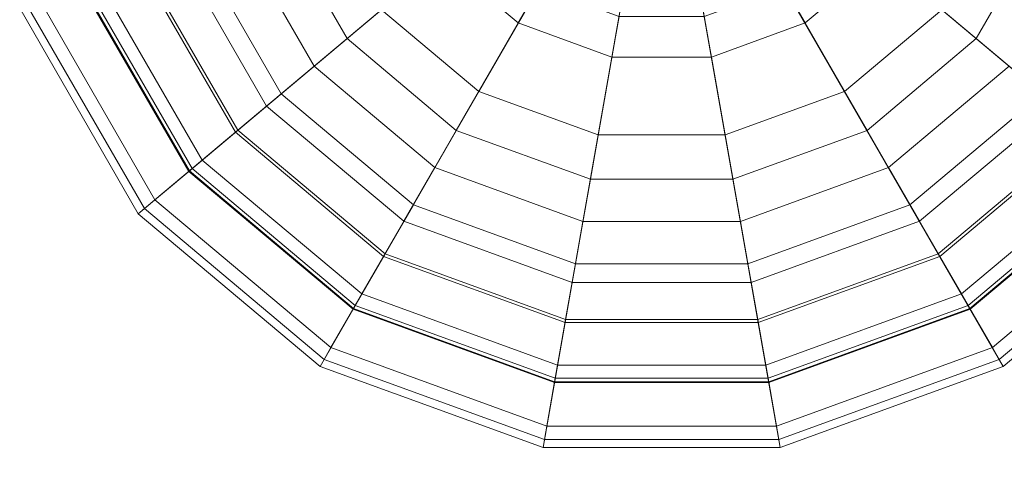
# Model space of a CAD drawing. Units: inches. Extents: x 375 to 1122, y 27 to 1069.
# Tile 30 of 155: x 731.789 to 733.741, y 279.842 to 280.756. Entities that reach past the tile are written whole.
import ezdxf

# ---------------------------------------------------------------- set-up
doc = ezdxf.new("R2010")
doc.units = ezdxf.units.IN
doc.layers.add('A-ANNO-DIMS', color=2, linetype='Continuous', lineweight=18)
doc.layers.add('Furniture', color=30, linetype='Continuous', lineweight=18)
doc.styles.get("Standard").update_dxf_attribs({"font": 'arial.ttf'})
doc.dimstyles.new('ISO-25', dxfattribs={"dimtxt": 12, "dimasz": 2.5, "dimexe": 1.5, "dimexo": 1.5, "dimtad": 1, "dimdec": 1, "dimlunit": 3, "dimtxsty": 'Standard', "dimblk": 'ARCHTICK', "dimcen": 2.5, "dimadec": 0, "dimazin": 0, "dimtfac": 1, "dimtdec": 1, "dimtmove": 0, "dimatfit": 3, "dimfxl": 1.5, "dimfxlon": 1, "dimarcsym": 0})

# ---------------------------------------------------------------- blocks, each defined once
blk = doc.blocks.new('A$C403C54AD')
for points in [[(1.64823, 1.228857, -0.04658), (1.626464, 1.202917, -0.043501), (1.626464, 1.202917, -0.043501), (1.638046, 1.234737, -0.04658)], [(1.635601, 1.213806, -0.040074), (1.646131, 1.226356, -0.043349), (1.636929, 1.231669, -0.043349), (1.631326, 1.216274, -0.040074)], [(1.65579, 1.219849, -0.04658), (1.626464, 1.202917, -0.043501), (1.626464, 1.202917, -0.043501), (1.64823, 1.228857, -0.04658)], [(1.652961, 1.218216, -0.043349), (1.65579, 1.219849, -0.04658), (1.64823, 1.228857, -0.04658), (1.646131, 1.226356, -0.043349)], [(1.644092, 1.223925, 0.056929), (1.63955, 1.218512, 0.046697), (1.633427, 1.222047, 0.046697), (1.635844, 1.228687, 0.056929)], [(1.652926, 1.218195, 0.116404), (1.655444, 1.219649, 0.10318), (1.647974, 1.228552, 0.10318), (1.646105, 1.226325, 0.116404)], [(1.655444, 1.219649, 0.10318), (1.65486, 1.219312, 0.074938), (1.64754, 1.228035, 0.074938), (1.647974, 1.228552, 0.10318)], [(1.65486, 1.219312, 0.074938), (1.650214, 1.216629, 0.056929), (1.644092, 1.223925, 0.056929), (1.64754, 1.228035, 0.074938)], [(1.638116, 1.216804, 0.048884), (1.642285, 1.221772, 0.058276), (1.634882, 1.226046, 0.058276), (1.632664, 1.219951, 0.048884)], [(1.638774, 1.210025, -0.040074), (1.652961, 1.218216, -0.043349), (1.646131, 1.226356, -0.043349), (1.635601, 1.213806, -0.040074)], [(1.648599, 1.215697, 0.12581), (1.652926, 1.218195, 0.116404), (1.646105, 1.226325, 0.116404), (1.642894, 1.222497, 0.12581)], [(1.652773, 1.218107, 0.102963), (1.65034, 1.216702, 0.115599), (1.644185, 1.224037, 0.115599), (1.645991, 1.226189, 0.102963)], [(1.652203, 1.217778, 0.075423), (1.652773, 1.218107, 0.102963), (1.645991, 1.226189, 0.102963), (1.645568, 1.225685, 0.075423)], [(1.64778, 1.215224, 0.058276), (1.652203, 1.217778, 0.075423), (1.645568, 1.225685, 0.075423), (1.642285, 1.221772, 0.058276)], [(1.65034, 1.216702, 0.115599), (1.645933, 1.214158, 0.12581), (1.640915, 1.220139, 0.12581), (1.644185, 1.224037, 0.115599)], [(1.650214, 1.216629, 0.056929), (1.644094, 1.213096, 0.046697), (1.63955, 1.218512, 0.046697), (1.644092, 1.223925, 0.056929)], [(1.63955, 1.218512, 0.046697), (1.632968, 1.210669, 0.03933), (1.629925, 1.212426, 0.03933), (1.633427, 1.222047, 0.046697)], [(1.645933, 1.214158, 0.12581), (1.648599, 1.215697, 0.12581), (1.642894, 1.222497, 0.12581), (1.640915, 1.220139, 0.12581)], [(1.642163, 1.211981, 0.048884), (1.64778, 1.215224, 0.058276), (1.642285, 1.221772, 0.058276), (1.638116, 1.216804, 0.048884)], [(1.659812, 1.208798, -0.04658), (1.626464, 1.202917, -0.043501), (1.626464, 1.202917, -0.043501), (1.65579, 1.219849, -0.04658)], [(1.656556, 1.208223, 0.116404), (1.659419, 1.208728, 0.10318), (1.655444, 1.219649, 0.10318), (1.652926, 1.218195, 0.116404)], [(1.656596, 1.20823, -0.043349), (1.659812, 1.208798, -0.04658), (1.65579, 1.219849, -0.04658), (1.652961, 1.218216, -0.043349)], [(1.659419, 1.208728, 0.10318), (1.658754, 1.208611, 0.074938), (1.65486, 1.219312, 0.074938), (1.655444, 1.219649, 0.10318)], [(1.658754, 1.208611, 0.074938), (1.653471, 1.20768, 0.056929), (1.650214, 1.216629, 0.056929), (1.65486, 1.219312, 0.074938)], [(1.644094, 1.213096, 0.046697), (1.635227, 1.207977, 0.03933), (1.632968, 1.210669, 0.03933), (1.63955, 1.218512, 0.046697)], [(1.640462, 1.205386, -0.040074), (1.656596, 1.20823, -0.043349), (1.652961, 1.218216, -0.043349), (1.638774, 1.210025, -0.040074)], [(1.651635, 1.207356, 0.12581), (1.656556, 1.208223, 0.116404), (1.652926, 1.218195, 0.116404), (1.648599, 1.215697, 0.12581)], [(1.650703, 1.207191, 0.058276), (1.655733, 1.208078, 0.075423), (1.652203, 1.217778, 0.075423), (1.64778, 1.215224, 0.058276)], [(1.656381, 1.208193, 0.102963), (1.653614, 1.207705, 0.115599), (1.65034, 1.216702, 0.115599), (1.652773, 1.218107, 0.102963)], [(1.655733, 1.208078, 0.075423), (1.656381, 1.208193, 0.102963), (1.652773, 1.218107, 0.102963), (1.652203, 1.217778, 0.075423)], [(1.634175, 1.207369, 0.042248), (1.642163, 1.211981, 0.048884), (1.638116, 1.216804, 0.048884), (1.632188, 1.209738, 0.042248)], [(1.653614, 1.207705, 0.115599), (1.648604, 1.206821, 0.12581), (1.645933, 1.214158, 0.12581), (1.65034, 1.216702, 0.115599)], [(1.653471, 1.20768, 0.056929), (1.646512, 1.206452, 0.046697), (1.644094, 1.213096, 0.046697), (1.650214, 1.216629, 0.056929)], [(1.648604, 1.206821, 0.12581), (1.651635, 1.207356, 0.12581), (1.648599, 1.215697, 0.12581), (1.645933, 1.214158, 0.12581)], [(1.644316, 1.206065, 0.048884), (1.650703, 1.207191, 0.058276), (1.64778, 1.215224, 0.058276), (1.642163, 1.211981, 0.048884)], [(1.637001, 1.209001, -0.037209), (1.638774, 1.210025, -0.040074), (1.635601, 1.213806, -0.040074), (1.634285, 1.212238, -0.037209)], [(1.646512, 1.206452, 0.046697), (1.636429, 1.204675, 0.03933), (1.635227, 1.207977, 0.03933), (1.644094, 1.213096, 0.046697)], [(1.635233, 1.204464, 0.042248), (1.644316, 1.206065, 0.048884), (1.642163, 1.211981, 0.048884), (1.634175, 1.207369, 0.042248)], [(1.638446, 1.20503, -0.037209), (1.640462, 1.205386, -0.040074), (1.638774, 1.210025, -0.040074), (1.637001, 1.209001, -0.037209)], [(1.659812, 1.197037, -0.04658), (1.626464, 1.202917, -0.043501), (1.626464, 1.202917, -0.043501), (1.659812, 1.208798, -0.04658)], [(1.658754, 1.197224, 0.074938), (1.653471, 1.198155, 0.056929), (1.653471, 1.20768, 0.056929), (1.658754, 1.208611, 0.074938)], [(1.656556, 1.197611, 0.116404), (1.659419, 1.197107, 0.10318), (1.659419, 1.208728, 0.10318), (1.656556, 1.208223, 0.116404)], [(1.656596, 1.197604, -0.043349), (1.659812, 1.197037, -0.04658), (1.659812, 1.208798, -0.04658), (1.656596, 1.20823, -0.043349)], [(1.659419, 1.197107, 0.10318), (1.658754, 1.197224, 0.074938), (1.658754, 1.208611, 0.074938), (1.659419, 1.208728, 0.10318)], [(1.640462, 1.200449, -0.040074), (1.656596, 1.197604, -0.043349), (1.656596, 1.20823, -0.043349), (1.640462, 1.205386, -0.040074)], [(1.650703, 1.198643, 0.058276), (1.655733, 1.197756, 0.075423), (1.655733, 1.208078, 0.075423), (1.650703, 1.207191, 0.058276)], [(1.651635, 1.198479, 0.12581), (1.656556, 1.197611, 0.116404), (1.656556, 1.208223, 0.116404), (1.651635, 1.207356, 0.12581)], [(1.656381, 1.197642, 0.102963), (1.653614, 1.19813, 0.115599), (1.653614, 1.207705, 0.115599), (1.656381, 1.208193, 0.102963)], [(1.655733, 1.197756, 0.075423), (1.656381, 1.197642, 0.102963), (1.656381, 1.208193, 0.102963), (1.655733, 1.208078, 0.075423)], [(1.653471, 1.198155, 0.056929), (1.646512, 1.199382, 0.046697), (1.646512, 1.206452, 0.046697), (1.653471, 1.20768, 0.056929)], [(1.653614, 1.19813, 0.115599), (1.648604, 1.199014, 0.12581), (1.648604, 1.206821, 0.12581), (1.653614, 1.207705, 0.115599)], [(1.644316, 1.19977, 0.048884), (1.650703, 1.198643, 0.058276), (1.650703, 1.207191, 0.058276), (1.644316, 1.206065, 0.048884)], [(1.648604, 1.199014, 0.12581), (1.651635, 1.198479, 0.12581), (1.651635, 1.207356, 0.12581), (1.648604, 1.206821, 0.12581)], [(1.646512, 1.199382, 0.046697), (1.636429, 1.20116, 0.03933), (1.636429, 1.204675, 0.03933), (1.646512, 1.206452, 0.046697)], [(1.635233, 1.201371, 0.042248), (1.644316, 1.19977, 0.048884), (1.644316, 1.206065, 0.048884), (1.635233, 1.204464, 0.042248)], [(1.638446, 1.200805, -0.037209), (1.640462, 1.200449, -0.040074), (1.640462, 1.205386, -0.040074), (1.638446, 1.20503, -0.037209)], [(1.65579, 1.185986, -0.04658), (1.626464, 1.202917, -0.043501), (1.626464, 1.202917, -0.043501), (1.659812, 1.197037, -0.04658)], [(1.64823, 1.176977, -0.04658), (1.626464, 1.202917, -0.043501), (1.626464, 1.202917, -0.043501), (1.65579, 1.185986, -0.04658)], [(1.638046, 1.171097, -0.04658), (1.626464, 1.202917, -0.043501), (1.626464, 1.202917, -0.043501), (1.64823, 1.176977, -0.04658)], [(1.634175, 1.198465, 0.042248), (1.642163, 1.193854, 0.048884), (1.644316, 1.19977, 0.048884), (1.635233, 1.201371, 0.042248)], [(1.644094, 1.192739, 0.046697), (1.635227, 1.197858, 0.03933), (1.636429, 1.20116, 0.03933), (1.646512, 1.199382, 0.046697)], [(1.637001, 1.196834, -0.037209), (1.638774, 1.19581, -0.040074), (1.640462, 1.200449, -0.040074), (1.638446, 1.200805, -0.037209)], [(1.638774, 1.19581, -0.040074), (1.652961, 1.187619, -0.043349), (1.656596, 1.197604, -0.043349), (1.640462, 1.200449, -0.040074)], [(1.642163, 1.193854, 0.048884), (1.64778, 1.190611, 0.058276), (1.650703, 1.198643, 0.058276), (1.644316, 1.19977, 0.048884)], [(1.650214, 1.189206, 0.056929), (1.644094, 1.192739, 0.046697), (1.646512, 1.199382, 0.046697), (1.653471, 1.198155, 0.056929)], [(1.645933, 1.191677, 0.12581), (1.648599, 1.190138, 0.12581), (1.651635, 1.198479, 0.12581), (1.648604, 1.199014, 0.12581)], [(1.65034, 1.189133, 0.115599), (1.645933, 1.191677, 0.12581), (1.648604, 1.199014, 0.12581), (1.653614, 1.19813, 0.115599)], [(1.64778, 1.190611, 0.058276), (1.652203, 1.188057, 0.075423), (1.655733, 1.197756, 0.075423), (1.650703, 1.198643, 0.058276)], [(1.632188, 1.196096, 0.042248), (1.638116, 1.189031, 0.048884), (1.642163, 1.193854, 0.048884), (1.634175, 1.198465, 0.042248)], [(1.648599, 1.190138, 0.12581), (1.652926, 1.187639, 0.116404), (1.656556, 1.197611, 0.116404), (1.651635, 1.198479, 0.12581)], [(1.65486, 1.186523, 0.074938), (1.650214, 1.189206, 0.056929), (1.653471, 1.198155, 0.056929), (1.658754, 1.197224, 0.074938)], [(1.652773, 1.187728, 0.102963), (1.65034, 1.189133, 0.115599), (1.653614, 1.19813, 0.115599), (1.656381, 1.197642, 0.102963)], [(1.63955, 1.187323, 0.046697), (1.632968, 1.195166, 0.03933), (1.635227, 1.197858, 0.03933), (1.644094, 1.192739, 0.046697)], [(1.652203, 1.188057, 0.075423), (1.652773, 1.187728, 0.102963), (1.656381, 1.197642, 0.102963), (1.655733, 1.197756, 0.075423)], [(1.652926, 1.187639, 0.116404), (1.655444, 1.186186, 0.10318), (1.659419, 1.197107, 0.10318), (1.656556, 1.197611, 0.116404)], [(1.652961, 1.187619, -0.043349), (1.65579, 1.185986, -0.04658), (1.659812, 1.197037, -0.04658), (1.656596, 1.197604, -0.043349)], [(1.655444, 1.186186, 0.10318), (1.65486, 1.186523, 0.074938), (1.658754, 1.197224, 0.074938), (1.659419, 1.197107, 0.10318)], [(1.634285, 1.193597, -0.037209), (1.635601, 1.192029, -0.040074), (1.638774, 1.19581, -0.040074), (1.637001, 1.196834, -0.037209)], [(1.635601, 1.192029, -0.040074), (1.646131, 1.179479, -0.043349), (1.652961, 1.187619, -0.043349), (1.638774, 1.19581, -0.040074)], [(1.633427, 1.183788, 0.046697), (1.629925, 1.193409, 0.03933), (1.632968, 1.195166, 0.03933), (1.63955, 1.187323, 0.046697)], [(1.638116, 1.189031, 0.048884), (1.642285, 1.184063, 0.058276), (1.64778, 1.190611, 0.058276), (1.642163, 1.193854, 0.048884)], [(1.644092, 1.18191, 0.056929), (1.63955, 1.187323, 0.046697), (1.644094, 1.192739, 0.046697), (1.650214, 1.189206, 0.056929)], [(1.631326, 1.18956, -0.040074), (1.636929, 1.174166, -0.043349), (1.646131, 1.179479, -0.043349), (1.635601, 1.192029, -0.040074)], [(1.640915, 1.185696, 0.12581), (1.642894, 1.183338, 0.12581), (1.648599, 1.190138, 0.12581), (1.645933, 1.191677, 0.12581)], [(1.644185, 1.181798, 0.115599), (1.640915, 1.185696, 0.12581), (1.645933, 1.191677, 0.12581), (1.65034, 1.189133, 0.115599)], [(1.642285, 1.184063, 0.058276), (1.645568, 1.18015, 0.075423), (1.652203, 1.188057, 0.075423), (1.64778, 1.190611, 0.058276)], [(1.642894, 1.183338, 0.12581), (1.646105, 1.17951, 0.116404), (1.652926, 1.187639, 0.116404), (1.648599, 1.190138, 0.12581)], [(1.632664, 1.185883, 0.048884), (1.634882, 1.179789, 0.058276), (1.642285, 1.184063, 0.058276), (1.638116, 1.189031, 0.048884)], [(1.64754, 1.1778, 0.074938), (1.644092, 1.18191, 0.056929), (1.650214, 1.189206, 0.056929), (1.65486, 1.186523, 0.074938)], [(1.645991, 1.179646, 0.102963), (1.644185, 1.181798, 0.115599), (1.65034, 1.189133, 0.115599), (1.652773, 1.187728, 0.102963)], [(1.645568, 1.18015, 0.075423), (1.645991, 1.179646, 0.102963), (1.652773, 1.187728, 0.102963), (1.652203, 1.188057, 0.075423)], [(1.646105, 1.17951, 0.116404), (1.647974, 1.177283, 0.10318), (1.655444, 1.186186, 0.10318), (1.652926, 1.187639, 0.116404)], [(1.646131, 1.179479, -0.043349), (1.64823, 1.176977, -0.04658), (1.65579, 1.185986, -0.04658), (1.652961, 1.187619, -0.043349)], [(1.635844, 1.177147, 0.056929), (1.633427, 1.183788, 0.046697), (1.63955, 1.187323, 0.046697), (1.644092, 1.18191, 0.056929)], [(1.647974, 1.177283, 0.10318), (1.64754, 1.1778, 0.074938), (1.65486, 1.186523, 0.074938), (1.655444, 1.186186, 0.10318)], [(1.634153, 1.181792, 0.12581), (1.635206, 1.178899, 0.12581), (1.642894, 1.183338, 0.12581), (1.640915, 1.185696, 0.12581)], [(1.635893, 1.177011, 0.115599), (1.634153, 1.181792, 0.12581), (1.640915, 1.185696, 0.12581), (1.644185, 1.181798, 0.115599)], [(1.634882, 1.179789, 0.058276), (1.636629, 1.174989, 0.075423), (1.645568, 1.18015, 0.075423), (1.642285, 1.184063, 0.058276)], [(1.635206, 1.178899, 0.12581), (1.636915, 1.174204, 0.116404), (1.646105, 1.17951, 0.116404), (1.642894, 1.183338, 0.12581)], [(1.637678, 1.172106, 0.074938), (1.635844, 1.177147, 0.056929), (1.644092, 1.18191, 0.056929), (1.64754, 1.1778, 0.074938)], [(1.636854, 1.174371, 0.102963), (1.635893, 1.177011, 0.115599), (1.644185, 1.181798, 0.115599), (1.645991, 1.179646, 0.102963)], [(1.636629, 1.174989, 0.075423), (1.636854, 1.174371, 0.102963), (1.645991, 1.179646, 0.102963), (1.645568, 1.18015, 0.075423)], [(1.636915, 1.174204, 0.116404), (1.637909, 1.171472, 0.10318), (1.647974, 1.177283, 0.10318), (1.646105, 1.17951, 0.116404)], [(1.636929, 1.174166, -0.043349), (1.638046, 1.171097, -0.04658), (1.64823, 1.176977, -0.04658), (1.646131, 1.179479, -0.043349)], [(1.637909, 1.171472, 0.10318), (1.637678, 1.172106, 0.074938), (1.64754, 1.1778, 0.074938), (1.647974, 1.177283, 0.10318)]]:
    blk.add_3dface(points)
blk = doc.blocks.new('_ArchTick')
at = {"color": 0, "linetype": 'ByBlock', "const_width": 0.15}
blk.add_lwpolyline([(-0.5, -0.5), (0.5, 0.5)], dxfattribs=at)
blk = doc.blocks.new('*D94')
at = {"layer": 'A-ANNO-DIMS', "color": 0, "lineweight": -2, "transparency": 16777216}
for p, q in [((734.0073, 117.5277), (734.0073, 114.5277)), ((773.0073, 117.5277), (773.0073, 114.5277)), ((734.0073, 116.0277), (773.0073, 116.0277))]:
    blk.add_line(p, q, dxfattribs=at)
at = {"layer": 'Defpoints', "color": 0, "transparency": 16777216}
for p in [(734.0073, 667.5277), (773.0073, 667.5277), (773.0073, 116.0277)]:
    blk.add_point(p, dxfattribs=at)
at = {"layer": 'A-ANNO-DIMS', "color": 0, "lineweight": -2, "transparency": 16777216, "xscale": 2.5, "yscale": 2.5, "zscale": 2.5, "rotation": 180}
blk.add_blockref('_ArchTick', (734.0073, 116.0277), dxfattribs=at)
at = {"layer": 'A-ANNO-DIMS', "color": 0, "lineweight": -2, "transparency": 16777216, "xscale": 2.5, "yscale": 2.5, "zscale": 2.5}
blk.add_blockref('_ArchTick', (773.0073, 116.0277), dxfattribs=at)
at = {"layer": 'A-ANNO-DIMS', "color": 0, "transparency": 16777216, "insert": (753.5073, 122.7837), "char_height": 12, "attachment_point": 5}
blk.add_mtext('3\'-3"', dxfattribs=at)

msp = doc.modelspace()

# ---------------------------------------------------------------- block references
at = {"layer": 'Furniture', "xscale": 39.9918517141215, "yscale": 39.9918517141215, "zscale": 39.9918517141215, "rotation": 270}
msp.add_blockref('A$C403C54AD', (684.9549, 346.2875, 0.024), dxfattribs=at)

# ---------------------------------------------------------------- dimensions: what is measured, and where the dimension line sits
at = {"layer": 'A-ANNO-DIMS'}
dim = msp.add_linear_dim(base=(773.0073, 116.0277), p1=(734.0073, 667.5277), p2=(773.0073, 667.5277), dimstyle='ISO-25', override={"dimdec": 1, "dimlfac": 1, "dimrnd": 0, "dimzin": 1, "dimdsep": 46, "dimlunit": 4, "dimfrac": 2}, dxfattribs=at)
dim.commit()
dim.dimension.update_dxf_attribs({"geometry": '*D94', "text_midpoint": (753.5073, 122.7837)})

doc.saveas('drawing.dxf')
